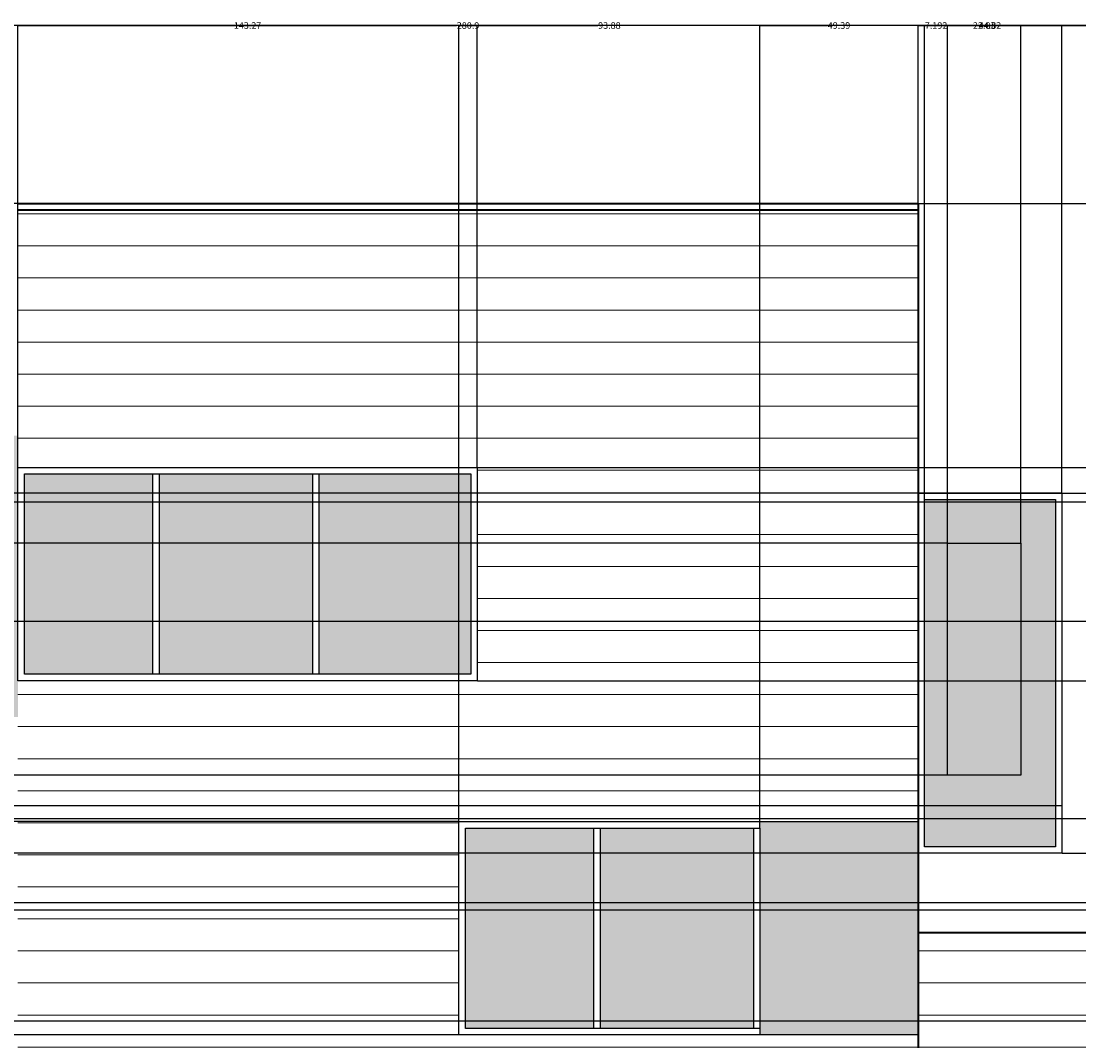
# Model space of a CAD drawing. Units: inches. Extents: x -30 to 1188, y 40 to 520.
# Tile 6 of 7: x 656 to 986, y 202 to 520. Entities that reach past the tile are written whole.
import ezdxf

# ---------------------------------------------------------------- set-up
doc = ezdxf.new("R2010")
doc.units = ezdxf.units.IN
doc.header["$MEASUREMENT"] = 0
for name, color, linetype, lineweight in [('A-ANNO-DIMS', 2, 'Continuous', 18), ('A-ELEV', 7, 'Continuous', 35), ('A-ELEV-PATT', 8, 'Continuous', 13), ('A-GLAZ', 4, 'Continuous', 25)]:
    doc.layers.add(name, color=color, linetype=linetype, lineweight=lineweight)
doc.styles.get("Standard").update_dxf_attribs({"font": 'arial.ttf'})
doc.dimstyles.get("Standard").update_dxf_attribs({"dimtxt": 2.0625, "dimasz": 0.18, "dimexe": 0.18, "dimexo": 0.0625, "dimgap": 0.09, "dimtad": 0, "dimtih": 1, "dimtoh": 1, "dimdec": 4, "dimzin": 0, "dimdsep": 46, "dimlunit": 4, "dimtxsty": 'Standard', "dimcen": 0.09, "dimadec": 0, "dimazin": 0, "dimtfac": 1, "dimtdec": 4, "dimtofl": 0, "dimtmove": 0, "dimatfit": 3, "dimfxl": 1, "dimtolj": 1, "dimtzin": 0, "dimarcsym": 0})

# ---------------------------------------------------------------- blocks, each defined once
blk = doc.blocks.new('*D7')
at = {"layer": 'A-ANNO-DIMS', "color": 0, "lineweight": -2, "transparency": 16777216}
for p, q in [((655.03, 463.36), (655.03, 518.97)), ((655.21, 518.79), (791.88, 518.79)), ((935.72, 518.79), (799.06, 518.79)), ((935.9, 463.36), (935.9, 518.97))]:
    blk.add_line(p, q, dxfattribs=at)
at = {"layer": 'A-ANNO-DIMS', "color": 0, "transparency": 16777216}
for points in [[(655.21, 518.82), (655.21, 518.76), (655.03, 518.79)], [(935.72, 518.82), (935.72, 518.76), (935.9, 518.79)]]:
    blk.add_solid(points, dxfattribs=at)
at = {"layer": 'Defpoints', "color": 0, "transparency": 16777216}
for p in [(935.9, 518.79), (655.03, 463.29), (935.9, 463.29)]:
    blk.add_point(p, dxfattribs=at)
at = {"layer": 'A-ANNO-DIMS', "color": 0, "transparency": 16777216, "insert": (795.47, 518.79), "char_height": 2.062, "attachment_point": 5}
blk.add_mtext('\\A1;280.9', dxfattribs=at)
blk = doc.blocks.new('*D8')
at = {"layer": 'A-ANNO-DIMS', "color": 0, "lineweight": -2, "transparency": 16777216}
for p, q in [((935.9, 235.79), (935.9, 518.97)), ((936.08, 518.79), (1017.62, 518.79)), ((1107.7, 518.79), (1026.16, 518.79)), ((1107.88, 235.79), (1107.88, 518.97))]:
    blk.add_line(p, q, dxfattribs=at)
at = {"layer": 'A-ANNO-DIMS', "color": 0, "transparency": 16777216}
for points in [[(936.08, 518.82), (936.08, 518.76), (935.9, 518.79)], [(1107.7, 518.82), (1107.7, 518.76), (1107.88, 518.79)]]:
    blk.add_solid(points, dxfattribs=at)
at = {"layer": 'Defpoints', "color": 0, "transparency": 16777216}
for p in [(1107.88, 518.79), (935.9, 235.73), (1107.88, 235.73)]:
    blk.add_point(p, dxfattribs=at)
at = {"layer": 'A-ANNO-DIMS', "color": 0, "transparency": 16777216, "insert": (1021.89, 518.79), "char_height": 2.062, "attachment_point": 5}
blk.add_mtext('\\A1;171.97', dxfattribs=at)
blk = doc.blocks.new('*D22')
at = {"layer": 'A-ANNO-DIMS', "color": 0, "lineweight": -2, "transparency": 16777216}
for p, q in [((935.9, 372.89), (935.9, 518.97)), ((936.08, 518.79), (954.71, 518.79)), ((980.55, 518.79), (961.92, 518.79)), ((980.73, 372.89), (980.73, 518.97))]:
    blk.add_line(p, q, dxfattribs=at)
at = {"layer": 'A-ANNO-DIMS', "color": 0, "transparency": 16777216}
for points in [[(936.08, 518.82), (936.08, 518.76), (935.9, 518.79)], [(980.55, 518.82), (980.55, 518.76), (980.73, 518.79)]]:
    blk.add_solid(points, dxfattribs=at)
at = {"layer": 'Defpoints', "color": 0, "transparency": 16777216}
for p in [(980.73, 518.79), (935.9, 372.83), (980.73, 372.83)]:
    blk.add_point(p, dxfattribs=at)
at = {"layer": 'A-ANNO-DIMS', "color": 0, "transparency": 16777216, "insert": (958.31, 518.79), "char_height": 2.062, "attachment_point": 5}
blk.add_mtext('\\A1;44.82', dxfattribs=at)
blk = doc.blocks.new('*D23')
at = {"layer": 'A-ANNO-DIMS', "color": 0, "lineweight": -2, "transparency": 16777216}
for p, q in [((980.79, 372.83), (1183.93, 372.83)), ((1183.75, 372.65), (1183.75, 317.8)), ((1183.75, 260.67), (1183.75, 315.52)), ((980.79, 260.49), (1183.93, 260.49))]:
    blk.add_line(p, q, dxfattribs=at)
at = {"layer": 'A-ANNO-DIMS', "color": 0, "transparency": 16777216}
for points in [[(1183.72, 372.65), (1183.78, 372.65), (1183.75, 372.83)], [(1183.72, 260.67), (1183.78, 260.67), (1183.75, 260.49)]]:
    blk.add_solid(points, dxfattribs=at)
at = {"layer": 'Defpoints', "color": 0, "transparency": 16777216}
for p in [(980.73, 372.83), (1183.75, 372.83), (980.73, 260.49)]:
    blk.add_point(p, dxfattribs=at)
at = {"layer": 'A-ANNO-DIMS', "color": 0, "transparency": 16777216, "insert": (1183.75, 316.66), "char_height": 2.062, "attachment_point": 5}
blk.add_mtext('\\A1;112.34', dxfattribs=at)
blk = doc.blocks.new('*D24')
at = {"layer": 'A-ANNO-DIMS', "color": 0, "lineweight": -2, "transparency": 16777216}
for p, q in [((935.84, 463.29), (-25.83, 463.29)), ((-25.65, 463.11), (-25.65, 419.2)), ((-25.65, 373.01), (-25.65, 416.92)), ((980.66, 372.83), (-25.83, 372.83))]:
    blk.add_line(p, q, dxfattribs=at)
at = {"layer": 'A-ANNO-DIMS', "color": 0, "transparency": 16777216}
for points in [[(-25.68, 463.11), (-25.62, 463.11), (-25.65, 463.29)], [(-25.68, 373.01), (-25.62, 373.01), (-25.65, 372.83)]]:
    blk.add_solid(points, dxfattribs=at)
at = {"layer": 'Defpoints', "color": 0, "transparency": 16777216}
for p in [(-25.65, 463.29), (935.9, 463.29), (980.73, 372.83)]:
    blk.add_point(p, dxfattribs=at)
at = {"layer": 'A-ANNO-DIMS', "color": 0, "transparency": 16777216, "insert": (-25.65, 418.06), "char_height": 2.062, "attachment_point": 5}
blk.add_mtext('\\A1;90.47', dxfattribs=at)
blk = doc.blocks.new('*D25')
at = {"layer": 'A-ANNO-DIMS', "color": 0, "lineweight": -2, "transparency": 16777216}
for p, q in [((655.03, 380.92), (655.03, 518.97)), ((655.21, 518.79), (722.39, 518.79)), ((798.12, 518.79), (730.94, 518.79)), ((798.3, 380.92), (798.3, 518.97))]:
    blk.add_line(p, q, dxfattribs=at)
at = {"layer": 'A-ANNO-DIMS', "color": 0, "transparency": 16777216}
for points in [[(655.21, 518.82), (655.21, 518.76), (655.03, 518.79)], [(798.12, 518.82), (798.12, 518.76), (798.3, 518.79)]]:
    blk.add_solid(points, dxfattribs=at)
at = {"layer": 'Defpoints', "color": 0, "transparency": 16777216}
for p in [(798.3, 518.79), (655.03, 380.86), (798.3, 380.86)]:
    blk.add_point(p, dxfattribs=at)
at = {"layer": 'A-ANNO-DIMS', "color": 0, "transparency": 16777216, "insert": (726.67, 518.79), "char_height": 2.062, "attachment_point": 5}
blk.add_mtext('\\A1;143.27', dxfattribs=at)
blk = doc.blocks.new('*D26')
at = {"layer": 'A-ANNO-DIMS', "color": 0, "lineweight": -2, "transparency": 16777216}
for p, q in [((798.37, 380.86), (1183.93, 380.86)), ((1183.75, 380.68), (1183.75, 348.74)), ((1183.75, 314.51), (1183.75, 346.45)), ((798.37, 314.33), (1183.93, 314.33))]:
    blk.add_line(p, q, dxfattribs=at)
at = {"layer": 'A-ANNO-DIMS', "color": 0, "transparency": 16777216}
for points in [[(1183.72, 380.68), (1183.78, 380.68), (1183.75, 380.86)], [(1183.72, 314.51), (1183.78, 314.51), (1183.75, 314.33)]]:
    blk.add_solid(points, dxfattribs=at)
at = {"layer": 'Defpoints', "color": 0, "transparency": 16777216}
for p in [(798.3, 380.86), (1183.75, 380.86), (798.3, 314.33)]:
    blk.add_point(p, dxfattribs=at)
at = {"layer": 'A-ANNO-DIMS', "color": 0, "transparency": 16777216, "insert": (1183.75, 347.6), "char_height": 2.062, "attachment_point": 5}
blk.add_mtext('\\A1;66.53', dxfattribs=at)
blk = doc.blocks.new('*D27')
at = {"layer": 'A-ANNO-DIMS', "color": 0, "lineweight": -2, "transparency": 16777216}
for p, q in [((792.63, 270.43), (792.63, 518.97)), ((792.81, 518.79), (836, 518.79)), ((886.34, 518.79), (843.15, 518.79)), ((886.52, 270.43), (886.52, 518.97))]:
    blk.add_line(p, q, dxfattribs=at)
at = {"layer": 'A-ANNO-DIMS', "color": 0, "transparency": 16777216}
for points in [[(792.81, 518.82), (792.81, 518.76), (792.63, 518.79)], [(886.34, 518.82), (886.34, 518.76), (886.52, 518.79)]]:
    blk.add_solid(points, dxfattribs=at)
at = {"layer": 'Defpoints', "color": 0, "transparency": 16777216}
for p in [(886.52, 518.79), (792.63, 270.37), (886.52, 270.37)]:
    blk.add_point(p, dxfattribs=at)
at = {"layer": 'A-ANNO-DIMS', "color": 0, "transparency": 16777216, "insert": (839.57, 518.79), "char_height": 2.062, "attachment_point": 5}
blk.add_mtext('\\A1;93.88', dxfattribs=at)
blk = doc.blocks.new('*D28')
at = {"layer": 'A-ANNO-DIMS', "color": 0, "lineweight": -2, "transparency": 16777216}
for p, q in [((886.52, 270.43), (886.52, 518.97)), ((886.7, 518.79), (907.6, 518.79)), ((935.72, 518.79), (914.82, 518.79)), ((935.9, 270.43), (935.9, 518.97))]:
    blk.add_line(p, q, dxfattribs=at)
at = {"layer": 'A-ANNO-DIMS', "color": 0, "transparency": 16777216}
for points in [[(886.7, 518.82), (886.7, 518.76), (886.52, 518.79)], [(935.72, 518.82), (935.72, 518.76), (935.9, 518.79)]]:
    blk.add_solid(points, dxfattribs=at)
at = {"layer": 'Defpoints', "color": 0, "transparency": 16777216}
for p in [(935.9, 518.79), (886.52, 270.37), (935.9, 270.37)]:
    blk.add_point(p, dxfattribs=at)
at = {"layer": 'A-ANNO-DIMS', "color": 0, "transparency": 16777216, "insert": (911.21, 518.79), "char_height": 2.062, "attachment_point": 5}
blk.add_mtext('\\A1;49.39', dxfattribs=at)
blk = doc.blocks.new('*D29')
at = {"layer": 'A-ANNO-DIMS', "color": 0, "lineweight": -2, "transparency": 16777216}
for p, q in [((792.57, 270.37), (-25.83, 270.37)), ((-25.65, 270.19), (-25.65, 238.25)), ((-25.65, 204.02), (-25.65, 235.96)), ((792.57, 203.84), (-25.83, 203.84))]:
    blk.add_line(p, q, dxfattribs=at)
at = {"layer": 'A-ANNO-DIMS', "color": 0, "transparency": 16777216}
for points in [[(-25.68, 270.19), (-25.62, 270.19), (-25.65, 270.37)], [(-25.68, 204.02), (-25.62, 204.02), (-25.65, 203.84)]]:
    blk.add_solid(points, dxfattribs=at)
at = {"layer": 'Defpoints', "color": 0, "transparency": 16777216}
for p in [(-25.65, 270.37), (792.63, 270.37), (792.63, 203.84)]:
    blk.add_point(p, dxfattribs=at)
at = {"layer": 'A-ANNO-DIMS', "color": 0, "transparency": 16777216, "insert": (-25.65, 237.11), "char_height": 2.062, "attachment_point": 5}
blk.add_mtext('\\A1;66.53', dxfattribs=at)
blk = doc.blocks.new('*D30')
at = {"layer": 'A-ANNO-DIMS', "color": 0, "lineweight": -2, "transparency": 16777216}
for p, q in [((935.97, 463.29), (1183.93, 463.29)), ((1183.75, 463.11), (1183.75, 423.22)), ((1183.75, 381.04), (1183.75, 420.93)), ((798.37, 380.86), (1183.93, 380.86))]:
    blk.add_line(p, q, dxfattribs=at)
at = {"layer": 'A-ANNO-DIMS', "color": 0, "transparency": 16777216}
for points in [[(1183.72, 463.11), (1183.78, 463.11), (1183.75, 463.29)], [(1183.72, 381.04), (1183.78, 381.04), (1183.75, 380.86)]]:
    blk.add_solid(points, dxfattribs=at)
at = {"layer": 'Defpoints', "color": 0, "transparency": 16777216}
for p in [(935.9, 463.29), (1183.75, 463.29), (798.3, 380.86)]:
    blk.add_point(p, dxfattribs=at)
at = {"layer": 'A-ANNO-DIMS', "color": 0, "transparency": 16777216, "insert": (1183.75, 422.08), "char_height": 2.062, "attachment_point": 5}
blk.add_mtext('\\A1;82.43', dxfattribs=at)
blk = doc.blocks.new('*D31')
at = {"layer": 'A-ANNO-DIMS', "color": 0, "lineweight": -2, "transparency": 16777216}
for p, q in [((792.57, 203.84), (-25.83, 203.84)), ((-25.65, 203.66), (-25.65, 164.5)), ((-25.65, 123.05), (-25.65, 162.21)), ((935.84, 122.87), (-25.83, 122.87))]:
    blk.add_line(p, q, dxfattribs=at)
at = {"layer": 'A-ANNO-DIMS', "color": 0, "transparency": 16777216}
for points in [[(-25.68, 203.66), (-25.62, 203.66), (-25.65, 203.84)], [(-25.68, 123.05), (-25.62, 123.05), (-25.65, 122.87)]]:
    blk.add_solid(points, dxfattribs=at)
at = {"layer": 'Defpoints', "color": 0, "transparency": 16777216}
for p in [(792.63, 203.84), (-25.65, 122.87), (935.9, 122.87)]:
    blk.add_point(p, dxfattribs=at)
at = {"layer": 'A-ANNO-DIMS', "color": 0, "transparency": 16777216, "insert": (-25.65, 163.36), "char_height": 2.062, "attachment_point": 5}
blk.add_mtext('\\A1;80.97', dxfattribs=at)
blk = doc.blocks.new('*D38')
at = {"layer": 'A-ANNO-DIMS', "color": 0, "lineweight": -2, "transparency": 16777216}
for p, q in [((99.49, 242.87), (1183.93, 242.87)), ((1183.75, 242.69), (1183.75, 216.04)), ((1183.75, 187.11), (1183.75, 213.76)), ((99.49, 186.93), (1183.93, 186.93))]:
    blk.add_line(p, q, dxfattribs=at)
at = {"layer": 'A-ANNO-DIMS', "color": 0, "transparency": 16777216}
for points in [[(1183.72, 242.69), (1183.78, 242.69), (1183.75, 242.87)], [(1183.72, 187.11), (1183.78, 187.11), (1183.75, 186.93)]]:
    blk.add_solid(points, dxfattribs=at)
at = {"layer": 'Defpoints', "color": 0, "transparency": 16777216}
for p in [(99.43, 242.87), (1183.75, 242.87), (99.43, 186.93)]:
    blk.add_point(p, dxfattribs=at)
at = {"layer": 'A-ANNO-DIMS', "color": 0, "transparency": 16777216, "insert": (1183.75, 214.9), "char_height": 2.062, "attachment_point": 5}
blk.add_mtext('\\A1;55.94', dxfattribs=at)
blk = doc.blocks.new('*D40')
at = {"layer": 'A-ANNO-DIMS', "color": 0, "lineweight": -2, "transparency": 16777216}
for p, q in [((358.49, 242.87), (1183.93, 242.87)), ((1183.75, 242.69), (1183.75, 216.04)), ((1183.75, 187.11), (1183.75, 213.76)), ((358.49, 186.93), (1183.93, 186.93))]:
    blk.add_line(p, q, dxfattribs=at)
at = {"layer": 'A-ANNO-DIMS', "color": 0, "transparency": 16777216}
for points in [[(1183.72, 242.69), (1183.78, 242.69), (1183.75, 242.87)], [(1183.72, 187.11), (1183.78, 187.11), (1183.75, 186.93)]]:
    blk.add_solid(points, dxfattribs=at)
at = {"layer": 'Defpoints', "color": 0, "transparency": 16777216}
for p in [(358.42, 242.87), (1183.75, 242.87), (358.42, 186.93)]:
    blk.add_point(p, dxfattribs=at)
at = {"layer": 'A-ANNO-DIMS', "color": 0, "transparency": 16777216, "insert": (1183.75, 214.9), "char_height": 2.062, "attachment_point": 5}
blk.add_mtext('\\A1;55.94', dxfattribs=at)
blk = doc.blocks.new('*D42')
at = {"layer": 'A-ANNO-DIMS', "color": 0, "lineweight": -2, "transparency": 16777216}
for p, q in [((945.1, 357.34), (945.1, 518.97)), ((945.28, 518.79), (952.92, 518.79)), ((967.75, 518.79), (960.1, 518.79)), ((967.93, 357.34), (967.93, 518.97))]:
    blk.add_line(p, q, dxfattribs=at)
at = {"layer": 'A-ANNO-DIMS', "color": 0, "transparency": 16777216}
for points in [[(945.28, 518.82), (945.28, 518.76), (945.1, 518.79)], [(967.75, 518.82), (967.75, 518.76), (967.93, 518.79)]]:
    blk.add_solid(points, dxfattribs=at)
at = {"layer": 'Defpoints', "color": 0, "transparency": 16777216}
for p in [(967.93, 518.79), (945.1, 357.27), (967.93, 357.27)]:
    blk.add_point(p, dxfattribs=at)
at = {"layer": 'A-ANNO-DIMS', "color": 0, "transparency": 16777216, "insert": (956.51, 518.79), "char_height": 2.062, "attachment_point": 5}
blk.add_mtext('\\A1;22.83', dxfattribs=at)
blk = doc.blocks.new('*D43')
at = {"layer": 'A-ANNO-DIMS', "color": 0, "lineweight": -2, "transparency": 16777216}
for p, q in [((937.72, 518.79), (937.54, 518.79)), ((937.9, 370.89), (937.9, 518.97)), ((945.1, 357.34), (945.1, 518.97)), ((945.28, 518.79), (945.46, 518.79))]:
    blk.add_line(p, q, dxfattribs=at)
at = {"layer": 'A-ANNO-DIMS', "color": 0, "transparency": 16777216}
for points in [[(937.72, 518.82), (937.72, 518.76), (937.9, 518.79)], [(945.28, 518.82), (945.28, 518.76), (945.1, 518.79)]]:
    blk.add_solid(points, dxfattribs=at)
at = {"layer": 'Defpoints', "color": 0, "transparency": 16777216}
for p in [(945.1, 518.79), (937.9, 370.83), (945.1, 357.27)]:
    blk.add_point(p, dxfattribs=at)
at = {"layer": 'A-ANNO-DIMS', "color": 0, "transparency": 16777216, "insert": (941.5, 518.79), "char_height": 2.062, "attachment_point": 5}
blk.add_mtext('\\A1;7.192', dxfattribs=at)
blk = doc.blocks.new('*D44')
at = {"layer": 'A-ANNO-DIMS', "color": 0, "lineweight": -2, "transparency": 16777216}
for p, q in [((980.66, 275.34), (-25.83, 275.34)), ((-25.65, 275.16), (-25.65, 269.06)), ((-25.65, 260.67), (-25.65, 266.77)), ((980.66, 260.49), (-25.83, 260.49))]:
    blk.add_line(p, q, dxfattribs=at)
at = {"layer": 'A-ANNO-DIMS', "color": 0, "transparency": 16777216}
for points in [[(-25.68, 275.16), (-25.62, 275.16), (-25.65, 275.34)], [(-25.68, 260.67), (-25.62, 260.67), (-25.65, 260.49)]]:
    blk.add_solid(points, dxfattribs=at)
at = {"layer": 'Defpoints', "color": 0, "transparency": 16777216}
for p in [(-25.65, 275.34), (980.73, 275.34), (980.73, 260.49)]:
    blk.add_point(p, dxfattribs=at)
at = {"layer": 'A-ANNO-DIMS', "color": 0, "transparency": 16777216, "insert": (-25.65, 267.92), "char_height": 2.062, "attachment_point": 5}
blk.add_mtext('\\A1;14.85', dxfattribs=at)
blk = doc.blocks.new('*D45')
at = {"layer": 'A-ANNO-DIMS', "color": 0, "lineweight": -2, "transparency": 16777216}
for p, q in [((945.03, 284.84), (-25.83, 284.84)), ((-25.65, 284.66), (-25.65, 273.81)), ((-25.65, 260.67), (-25.65, 271.52)), ((935.84, 260.49), (-25.83, 260.49))]:
    blk.add_line(p, q, dxfattribs=at)
at = {"layer": 'A-ANNO-DIMS', "color": 0, "transparency": 16777216}
for points in [[(-25.68, 284.66), (-25.62, 284.66), (-25.65, 284.84)], [(-25.68, 260.67), (-25.62, 260.67), (-25.65, 260.49)]]:
    blk.add_solid(points, dxfattribs=at)
at = {"layer": 'Defpoints', "color": 0, "transparency": 16777216}
for p in [(945.1, 284.84), (-25.65, 260.49), (935.9, 260.49)]:
    blk.add_point(p, dxfattribs=at)
at = {"layer": 'A-ANNO-DIMS', "color": 0, "transparency": 16777216, "insert": (-25.65, 272.67), "char_height": 2.062, "attachment_point": 5}
blk.add_mtext('\\A1;24.35', dxfattribs=at)
blk = doc.blocks.new('*D46')
at = {"layer": 'A-ANNO-DIMS', "color": 0, "lineweight": -2, "transparency": 16777216}
for p, q in [((945.03, 357.27), (-25.83, 357.27)), ((-25.65, 357.09), (-25.65, 322.2)), ((-25.65, 285.02), (-25.65, 319.91)), ((945.03, 284.84), (-25.83, 284.84))]:
    blk.add_line(p, q, dxfattribs=at)
at = {"layer": 'A-ANNO-DIMS', "color": 0, "transparency": 16777216}
for points in [[(-25.68, 357.09), (-25.62, 357.09), (-25.65, 357.27)], [(-25.68, 285.02), (-25.62, 285.02), (-25.65, 284.84)]]:
    blk.add_solid(points, dxfattribs=at)
at = {"layer": 'Defpoints', "color": 0, "transparency": 16777216}
for p in [(-25.65, 357.27), (945.1, 357.27), (945.1, 284.84)]:
    blk.add_point(p, dxfattribs=at)
at = {"layer": 'A-ANNO-DIMS', "color": 0, "transparency": 16777216, "insert": (-25.65, 321.06), "char_height": 2.062, "attachment_point": 5}
blk.add_mtext('\\A1;72.43', dxfattribs=at)
blk = doc.blocks.new('*D47')
at = {"layer": 'A-ANNO-DIMS', "color": 0, "lineweight": -2, "transparency": 16777216}
for p, q in [((935.84, 372.83), (-25.83, 372.83)), ((-25.65, 372.65), (-25.65, 366.19)), ((-25.65, 357.45), (-25.65, 363.91)), ((945.03, 357.27), (-25.83, 357.27))]:
    blk.add_line(p, q, dxfattribs=at)
at = {"layer": 'A-ANNO-DIMS', "color": 0, "transparency": 16777216}
for points in [[(-25.68, 372.65), (-25.62, 372.65), (-25.65, 372.83)], [(-25.68, 357.45), (-25.62, 357.45), (-25.65, 357.27)]]:
    blk.add_solid(points, dxfattribs=at)
at = {"layer": 'Defpoints', "color": 0, "transparency": 16777216}
for p in [(-25.65, 372.83), (935.9, 372.83), (945.1, 357.27)]:
    blk.add_point(p, dxfattribs=at)
at = {"layer": 'A-ANNO-DIMS', "color": 0, "transparency": 16777216, "insert": (-25.65, 365.05), "char_height": 2.062, "attachment_point": 5}
blk.add_mtext('\\A1;15.554', dxfattribs=at)
blk = doc.blocks.new('*D61')
at = {"layer": 'A-ANNO-DIMS', "color": 0, "lineweight": -2, "transparency": 16777216}
for p, q in [((653.09, 208.22), (1183.93, 208.22)), ((1183.75, 208.04), (1183.75, 176.65)), ((1183.75, 142.98), (1183.75, 174.36)), ((652.92, 142.8), (1183.93, 142.8))]:
    blk.add_line(p, q, dxfattribs=at)
at = {"layer": 'A-ANNO-DIMS', "color": 0, "transparency": 16777216}
for points in [[(1183.72, 208.04), (1183.78, 208.04), (1183.75, 208.22)], [(1183.72, 142.98), (1183.78, 142.98), (1183.75, 142.8)]]:
    blk.add_solid(points, dxfattribs=at)
at = {"layer": 'Defpoints', "color": 0, "transparency": 16777216}
for p in [(653.03, 208.22), (1183.75, 208.22), (652.86, 142.8)]:
    blk.add_point(p, dxfattribs=at)
at = {"layer": 'A-ANNO-DIMS', "color": 0, "transparency": 16777216, "insert": (1183.75, 175.51), "char_height": 2.062, "attachment_point": 5}
blk.add_mtext('\\A1;65.42', dxfattribs=at)
blk = doc.blocks.new('*D62')
at = {"layer": 'A-ANNO-DIMS', "color": 0, "lineweight": -2, "transparency": 16777216}
for p, q in [((652.92, 271.38), (1183.93, 271.38)), ((1183.75, 271.2), (1183.75, 240.94)), ((1183.75, 208.4), (1183.75, 238.65)), ((653.09, 208.22), (1183.93, 208.22))]:
    blk.add_line(p, q, dxfattribs=at)
at = {"layer": 'A-ANNO-DIMS', "color": 0, "transparency": 16777216}
for points in [[(1183.72, 271.2), (1183.78, 271.2), (1183.75, 271.38)], [(1183.72, 208.4), (1183.78, 208.4), (1183.75, 208.22)]]:
    blk.add_solid(points, dxfattribs=at)
at = {"layer": 'Defpoints', "color": 0, "transparency": 16777216}
for p in [(652.86, 271.38), (1183.75, 271.38), (653.03, 208.22)]:
    blk.add_point(p, dxfattribs=at)
at = {"layer": 'A-ANNO-DIMS', "color": 0, "transparency": 16777216, "insert": (1183.75, 239.8), "char_height": 2.062, "attachment_point": 5}
blk.add_mtext('\\A1;63.16', dxfattribs=at)
blk = doc.blocks.new('*D64')
at = {"layer": 'A-ANNO-DIMS', "color": 0, "lineweight": -2, "transparency": 16777216}
for p, q in [((576.85, 245.17), (1183.93, 245.17)), ((1183.75, 244.99), (1183.75, 200.27)), ((1183.75, 153.26), (1183.75, 197.98)), ((576.85, 153.08), (1183.93, 153.08))]:
    blk.add_line(p, q, dxfattribs=at)
at = {"layer": 'A-ANNO-DIMS', "color": 0, "transparency": 16777216}
for points in [[(1183.72, 244.99), (1183.78, 244.99), (1183.75, 245.17)], [(1183.72, 153.26), (1183.78, 153.26), (1183.75, 153.08)]]:
    blk.add_solid(points, dxfattribs=at)
at = {"layer": 'Defpoints', "color": 0, "transparency": 16777216}
for p in [(576.78, 245.17), (1183.75, 245.17), (576.78, 153.08)]:
    blk.add_point(p, dxfattribs=at)
at = {"layer": 'A-ANNO-DIMS', "color": 0, "transparency": 16777216, "insert": (1183.75, 199.12), "char_height": 2.062, "attachment_point": 5}
blk.add_mtext('\\A1;92.08', dxfattribs=at)
blk = doc.blocks.new('*D68')
at = {"layer": 'A-ANNO-DIMS', "color": 0, "lineweight": -2, "transparency": 16777216}
for p, q in [((580.04, 370.13), (1183.93, 370.13)), ((1183.75, 369.95), (1183.75, 352.67)), ((1183.75, 333.09), (1183.75, 350.38)), ((580.04, 332.91), (1183.93, 332.91))]:
    blk.add_line(p, q, dxfattribs=at)
at = {"layer": 'A-ANNO-DIMS', "color": 0, "transparency": 16777216}
for points in [[(1183.72, 369.95), (1183.78, 369.95), (1183.75, 370.13)], [(1183.72, 333.09), (1183.78, 333.09), (1183.75, 332.91)]]:
    blk.add_solid(points, dxfattribs=at)
at = {"layer": 'Defpoints', "color": 0, "transparency": 16777216}
for p in [(579.97, 370.13), (1183.75, 370.13), (579.97, 332.91)]:
    blk.add_point(p, dxfattribs=at)
at = {"layer": 'A-ANNO-DIMS', "color": 0, "transparency": 16777216, "insert": (1183.75, 351.52), "char_height": 2.062, "attachment_point": 5}
blk.add_mtext('\\A1;37.22', dxfattribs=at)
blk = doc.blocks.new('*D74')
at = {"layer": 'A-ANNO-DIMS', "color": 0, "lineweight": -2, "transparency": 16777216}
for p, q in [((30.14, 98.93), (30.14, 518.97)), ((30.32, 518.79), (574.32, 518.79)), ((1128.07, 518.79), (584.07, 518.79)), ((1128.25, 117.62), (1128.25, 518.97))]:
    blk.add_line(p, q, dxfattribs=at)
at = {"layer": 'A-ANNO-DIMS', "color": 0, "transparency": 16777216}
for points in [[(30.32, 518.82), (30.32, 518.76), (30.14, 518.79)], [(1128.07, 518.82), (1128.07, 518.76), (1128.25, 518.79)]]:
    blk.add_solid(points, dxfattribs=at)
at = {"layer": 'Defpoints', "color": 0, "transparency": 16777216}
for p in [(1128.25, 518.79), (1128.25, 117.56), (30.14, 98.87)]:
    blk.add_point(p, dxfattribs=at)
at = {"layer": 'A-ANNO-DIMS', "color": 0, "transparency": 16777216, "insert": (579.19, 518.79), "char_height": 2.0625, "attachment_point": 5}
blk.add_mtext('\\A1;1098.11', dxfattribs=at)

msp = doc.modelspace()

# ---------------------------------------------------------------- hatches: boundary and pattern name
at = {"layer": 'A-ELEV-PATT'}
h = msp.add_hatch(dxfattribs=at)
h.set_pattern_fill('ANSI31', color=256, scale=80, angle=135)
h.paths.add_polyline_path([(935.904, 461.2934), (655.0318, 461.2934), (655.0318, 408.0708), (655.0318, 380.8615), (798.3036, 380.8615), (798.3036, 314.3348), (655.0318, 314.3348), (655.0318, 303.0545), (655.0318, 122.8714), (744.4225, 122.8714), (796.5546, 122.8714), (935.904, 122.8714), (935.904, 203.8438), (792.6322, 203.8438), (792.6322, 270.3705), (935.904, 270.3705), (935.904, 372.8284)])
h.paths.add_polyline_path([(466.9951, 434.8714), (466.9951, 461.2934), (73.6582, 461.2934), (73.6582, 434.8714), (73.6582, 410.8714), (73.6582, 266.8714), (382.4247, 266.8714), (466.9951, 266.8714)])
h.paths.add_polyline_path([(422.6392, 390.3227), (422.6392, 317.8826), (99.4312, 317.8826), (99.4312, 390.3227)], flags=16)
h.paths.add_polyline_path([(416.8376, 385.9009), (416.8376, 322.3026), (332.2885, 322.3026), (332.2885, 385.9009)], flags=0)
h.paths.add_polyline_path([(187.4151, 386.0591), (187.4151, 322.4608), (102.866, 322.4608), (102.866, 386.0591)], flags=0)
h = msp.add_hatch(color=256, dxfattribs=at)
h.dxf.hatch_style = 1
h.paths.add_polyline_path([(521.0073, 390.7733), (466.9951, 390.7733), (466.9951, 303.0545), (521.0073, 303.0545)])
h.paths.add_polyline_path([(588.0971, 390.7733), (523.0073, 390.7733), (523.0073, 303.0545), (588.0971, 303.0545)])
h.paths.add_polyline_path([(579.9749, 370.1304), (579.9749, 332.9128), (530.7254, 332.9128), (530.7254, 370.1304)], flags=16)
h.paths.add_polyline_path([(577.9749, 368.1304), (577.9749, 334.9128), (532.7254, 334.9128), (532.7254, 368.1304)], flags=0)
h.paths.add_polyline_path([(655.0318, 390.7733), (590.0971, 390.7733), (590.0971, 303.0545), (655.0318, 303.0545)])
h.paths.add_polyline_path([(577.9749, 368.1304), (532.7254, 368.1304), (532.7254, 334.9128), (577.9749, 334.9128)], flags=0)
h.paths.add_polyline_path([(416.8376, 385.9009), (374.5631, 385.9009), (374.5631, 322.3026), (416.8376, 322.3026)])
h.paths.add_polyline_path([(372.5631, 385.9009), (332.2885, 385.9009), (332.2885, 322.3026), (372.5631, 322.3026)])
h.paths.add_polyline_path([(187.4151, 386.0591), (102.866, 386.0591), (102.866, 322.4608), (187.4151, 322.4608)])
h.paths.add_polyline_path([(697.0557, 378.8615), (657.0318, 378.8615), (657.0318, 316.3348), (697.0557, 316.3348)])
h.paths.add_polyline_path([(746.916, 378.8615), (699.0557, 378.8615), (699.0557, 316.3348), (746.916, 316.3348)])
h.paths.add_polyline_path([(796.3036, 378.8615), (748.916, 378.8615), (748.916, 316.3348), (796.3036, 316.3348)])
h.paths.add_polyline_path([(884.5164, 268.3705), (836.6561, 268.3705), (836.6561, 205.8438), (884.5164, 205.8438)])
h.paths.add_polyline_path([(834.6561, 268.3705), (794.6322, 268.3705), (794.6322, 205.8438), (834.6561, 205.8438)])
h.paths.add_polyline_path([(967.928, 357.2748), (945.0964, 357.2748), (945.0964, 284.8425), (967.928, 284.8425)])
h = msp.add_hatch(color=256, dxfattribs=at)
h.dxf.hatch_style = 1
h.paths.add_polyline_path([(237.1312, 390.3227), (187.4151, 390.3227), (187.4151, 386.0591), (187.4151, 322.4608), (187.4151, 317.8826), (237.1312, 317.8826)])
h.paths.add_polyline_path([(289.6973, 390.3227), (237.1312, 390.3227), (237.1312, 317.8826), (289.6973, 317.8826)])
h.paths.add_polyline_path([(422.6392, 390.3227), (289.6973, 390.3227), (289.6973, 317.8826), (422.6392, 317.8826)])
h.paths.add_polyline_path([(332.2885, 385.9009), (416.8376, 385.9009), (416.8376, 322.3026), (332.2885, 322.3026)], flags=16)
h.paths.add_polyline_path([(520.8377, 255.4488), (468.8255, 255.4488), (468.8255, 208.218), (520.8377, 208.218)])
h.paths.add_polyline_path([(573.9028, 245.1654), (576.7826, 245.1654), (576.7826, 208.218), (587.9675, 208.218), (587.9675, 255.4488), (522.8377, 255.4488), (522.8377, 208.218), (573.9028, 208.218)])
h.paths.add_polyline_path([(652.8622, 255.4488), (589.9675, 255.4488), (589.9675, 208.218), (652.8622, 208.218)])
h.paths.add_polyline_path([(652.8622, 206.218), (589.9675, 206.218), (589.9675, 142.7981), (652.8622, 142.7981)])
h.paths.add_polyline_path([(573.9028, 206.218), (522.8377, 206.218), (522.8377, 142.7981), (587.9675, 142.7981), (587.9675, 206.218), (576.7826, 206.218), (576.7826, 153.0843), (573.9028, 153.0843)])
h.paths.add_polyline_path([(520.8377, 206.218), (468.8255, 206.218), (468.8255, 142.7981), (520.8377, 142.7981)])
h.paths.add_polyline_path([(520.8377, 271.3754), (468.8255, 271.3754), (468.8255, 255.4488), (520.8377, 255.4488)])
h.paths.add_polyline_path([(587.9675, 271.3754), (522.8377, 271.3754), (522.8377, 255.4488), (587.9675, 255.4488)])
h.paths.add_polyline_path([(652.8622, 271.3754), (589.9675, 271.3754), (589.9675, 255.4488), (652.8622, 255.4488)])
h.paths.add_polyline_path([(935.904, 270.3705), (886.5164, 270.3705), (886.5164, 268.3705), (886.5164, 205.8438), (886.5164, 203.8438), (935.904, 203.8438)])
h.paths.add_polyline_path([(978.7252, 275.3408), (937.904, 275.3408), (937.904, 262.4906), (978.7252, 262.4906)])
h.paths.add_polyline_path([(978.7252, 370.8284), (937.904, 370.8284), (937.904, 275.3408), (978.7252, 275.3408)])
h.paths.add_polyline_path([(967.928, 284.8425), (945.0964, 284.8425), (945.0964, 357.2748), (967.928, 357.2748)], flags=16)
h = msp.add_hatch(dxfattribs=at)
h.set_pattern_fill('ANSI31', color=256, scale=80, angle=135)
h.paths.add_polyline_path([(1107.8751, 235.7299), (935.904, 235.7299), (935.904, 122.8714), (995.9226, 122.8714), (1107.8751, 118.3767)])

# ---------------------------------------------------------------- linework, layer by layer
at = {"layer": 'A-ELEV'}
for p, q in [((655.0318, 463.2934), (935.904, 463.2934)), ((935.904, 463.2934), (935.904, 122.8714)), ((655.0318, 461.2934), (935.904, 461.2934)), ((935.904, 235.7299), (1107.8751, 235.7299))]:
    msp.add_line(p, q, dxfattribs=at)
at = {"layer": 'A-GLAZ'}
for p, q in [((697.0557, 378.8615), (697.0557, 316.3348)), ((699.0557, 378.8615), (699.0557, 316.3348)), ((746.916, 378.8615), (746.916, 316.3348)), ((748.916, 378.8615), (748.916, 316.3348)), ((937.904, 275.3408), (980.7252, 275.3408)), ((834.6561, 268.3705), (834.6561, 205.8438)), ((836.6561, 268.3705), (836.6561, 205.8438)), ((884.5164, 268.3705), (884.5164, 205.8438)), ((886.5164, 268.3705), (886.5164, 270.3705)), ((886.5164, 268.3705), (886.5164, 205.8438)), ((886.5164, 205.8438), (886.5164, 203.8438))]:
    msp.add_line(p, q, dxfattribs=at)
for points in [[(655.0318, 380.8615), (798.3036, 380.8615), (798.3036, 314.3348), (655.0318, 314.3348)], [(657.0318, 378.8615), (796.3036, 378.8615), (796.3036, 316.3348), (657.0318, 316.3348)], [(935.904, 372.8284), (980.7252, 372.8284), (980.7252, 260.4906), (935.904, 260.4906)], [(937.904, 370.8284), (978.7252, 370.8284), (978.7252, 262.4906), (937.904, 262.4906)], [(945.0964, 357.2748), (967.928, 357.2748), (967.928, 284.8425), (945.0964, 284.8425)], [(792.6322, 270.3705), (935.904, 270.3705), (935.904, 203.8438), (792.6322, 203.8438)], [(794.6322, 268.3705), (886.5164, 268.3705), (886.5164, 205.8438), (794.6322, 205.8438)]]:
    msp.add_lwpolyline(points, close=True, dxfattribs=at)

# ---------------------------------------------------------------- dimensions: what is measured, and where the dimension line sits
at = {"layer": 'A-ANNO-DIMS'}
for base, p1, p2, override, picture, middle in [((1128.2474, 518.7934), (30.1395, 98.8714), (1128.2474, 117.5588), {"dimdec": 2, "dimlfac": 1, "dimrnd": 0, "dimzin": 0, "dimdsep": 46, "dimlunit": 2}, '*D74', (579.1935, 518.7934)), ((935.904, 518.7934), (655.0318, 463.2934), (935.904, 463.2934), {"dimdec": 1, "dimlfac": 1, "dimrnd": 0, "dimzin": 0, "dimdsep": 46, "dimlunit": 2}, '*D7', (795.4679, 518.7934)), ((798.3036, 518.7934), (655.0318, 380.8615), (798.3036, 380.8615), {"dimdec": 2, "dimlfac": 1, "dimrnd": 0, "dimzin": 0, "dimdsep": 46, "dimlunit": 2}, '*D25', (726.6677, 518.7934)), ((886.5164, 518.7934), (792.6322, 270.3705), (886.5164, 270.3705), {"dimdec": 2, "dimlfac": 1, "dimrnd": 0, "dimzin": 0, "dimdsep": 46, "dimlunit": 2}, '*D27', (839.5743, 518.7934)), ((935.904, 518.7934), (886.5164, 270.3705), (935.904, 270.3705), {"dimdec": 2, "dimlfac": 1, "dimrnd": 0, "dimzin": 0, "dimdsep": 46, "dimlunit": 2}, '*D28', (911.2102, 518.7934)), ((1107.8751, 518.7934), (935.904, 235.7299), (1107.8751, 235.7299), {"dimdec": 2, "dimlfac": 1, "dimrnd": 0, "dimzin": 0, "dimdsep": 46, "dimlunit": 2}, '*D8', (1021.8896, 518.7934)), ((980.7252, 518.7934), (935.904, 372.8284), (980.7252, 372.8284), {"dimdec": 2, "dimlfac": 1, "dimrnd": 0, "dimzin": 0, "dimdsep": 46, "dimlunit": 2}, '*D22', (958.3146, 518.7934)), ((945.0964, 518.7934), (937.904, 370.8284), (945.0964, 357.2748), {"dimdec": 3, "dimlfac": 1, "dimrnd": 0, "dimzin": 0, "dimdsep": 46, "dimlunit": 2}, '*D43', (941.5002, 518.7934)), ((967.928, 518.7934), (945.0964, 357.2748), (967.928, 357.2748), {"dimdec": 2, "dimlfac": 1, "dimrnd": 0, "dimzin": 0, "dimdsep": 46, "dimlunit": 2}, '*D42', (956.5122, 518.7934))]:
    dim = msp.add_linear_dim(base=base, p1=p1, p2=p2, dimstyle='Standard', override=override, dxfattribs=at)
    dim.commit()
    dim.dimension.update_dxf_attribs({"geometry": picture, "text_midpoint": middle})
for base, p1, p2, override, picture, middle in [((-25.64838, 463.29342), (980.72519, 372.8284), (935.90404, 463.29342), {"dimdec": 2, "dimlfac": 1, "dimrnd": 0, "dimzin": 0, "dimdsep": 46, "dimlunit": 2}, '*D24', (-25.64838, 418.06091)), ((1183.7474, 463.2934), (798.3036, 380.8615), (935.904, 463.2934), {"dimdec": 2, "dimlfac": 1, "dimrnd": 0, "dimzin": 0, "dimdsep": 46, "dimlunit": 2}, '*D30', (1183.7474, 422.0775)), ((1183.7474, 380.8615), (798.3036, 314.3348), (798.3036, 380.8615), {"dimdec": 2, "dimlfac": 1, "dimrnd": 0, "dimzin": 0, "dimdsep": 46, "dimlunit": 2}, '*D26', (1183.7474, 347.5982)), ((-25.6484, 372.8284), (945.0964, 357.2748), (935.904, 372.8284), {"dimdec": 3, "dimlfac": 1, "dimrnd": 0, "dimzin": 0, "dimdsep": 46, "dimlunit": 2}, '*D47', (-25.6484, 365.0516)), ((1183.7474, 370.1304), (579.9749, 332.9128), (579.9749, 370.1304), {"dimdec": 2, "dimlfac": 1, "dimrnd": 0, "dimzin": 0, "dimdsep": 46, "dimlunit": 2}, '*D68', (1183.7474, 351.5216)), ((1183.7474, 372.8284), (980.7252, 260.4906), (980.7252, 372.8284), {"dimdec": 2, "dimlfac": 1, "dimrnd": 0, "dimzin": 0, "dimdsep": 46, "dimlunit": 2}, '*D23', (1183.7474, 316.6595)), ((-25.6484, 357.2748), (945.0964, 284.8425), (945.0964, 357.2748), {"dimdec": 2, "dimlfac": 1, "dimrnd": 0, "dimzin": 0, "dimdsep": 46, "dimlunit": 2}, '*D46', (-25.6484, 321.0586)), ((-25.6484, 260.4906), (945.0964, 284.8425), (935.904, 260.4906), {"dimdec": 2, "dimlfac": 1, "dimrnd": 0, "dimzin": 0, "dimdsep": 46, "dimlunit": 2}, '*D45', (-25.6484, 272.6666)), ((-25.6484, 275.3408), (980.7252, 260.4906), (980.7252, 275.3408), {"dimdec": 2, "dimlfac": 1, "dimrnd": 0, "dimzin": 0, "dimdsep": 46, "dimlunit": 2}, '*D44', (-25.6484, 267.9157)), ((1183.7474, 271.3754), (653.0318, 208.218), (652.8622, 271.3754), {"dimdec": 2, "dimlfac": 1, "dimrnd": 0, "dimzin": 0, "dimdsep": 46, "dimlunit": 2}, '*D62', (1183.7474, 239.7967)), ((-25.6484, 270.3705), (792.6322, 203.8438), (792.6322, 270.3705), {"dimdec": 2, "dimlfac": 1, "dimrnd": 0, "dimzin": 0, "dimdsep": 46, "dimlunit": 2}, '*D29', (-25.6484, 237.1071)), ((1183.7474, 245.1654), (576.7826, 153.0843), (576.7826, 245.1654), {"dimdec": 2, "dimlfac": 1, "dimrnd": 0, "dimzin": 0, "dimdsep": 46, "dimlunit": 2}, '*D64', (1183.7474, 199.1248)), ((1183.7474, 242.8714), (99.4312, 186.9265), (99.4312, 242.8714), {"dimdec": 2, "dimlfac": 1, "dimrnd": 0, "dimzin": 0, "dimdsep": 46, "dimlunit": 2}, '*D38', (1183.7474, 214.899)), ((1183.7474, 242.8714), (358.4247, 186.9265), (358.4247, 242.8714), {"dimdec": 2, "dimlfac": 1, "dimrnd": 0, "dimzin": 0, "dimdsep": 46, "dimlunit": 2}, '*D40', (1183.7474, 214.899)), ((1183.7474, 208.218), (652.8622, 142.7981), (653.0318, 208.218), {"dimdec": 2, "dimlfac": 1, "dimrnd": 0, "dimzin": 0, "dimdsep": 46, "dimlunit": 2}, '*D61', (1183.7474, 175.508)), ((-25.6484, 122.8714), (792.6322, 203.8438), (935.904, 122.8714), {"dimdec": 2, "dimlfac": 1, "dimrnd": 0, "dimzin": 0, "dimdsep": 46, "dimlunit": 2}, '*D31', (-25.6484, 163.3576))]:
    dim = msp.add_linear_dim(base=base, p1=p1, p2=p2, angle=90, dimstyle='Standard', override=override, dxfattribs=at)
    dim.commit()
    dim.dimension.update_dxf_attribs({"geometry": picture, "text_midpoint": middle})

doc.saveas('drawing.dxf')
